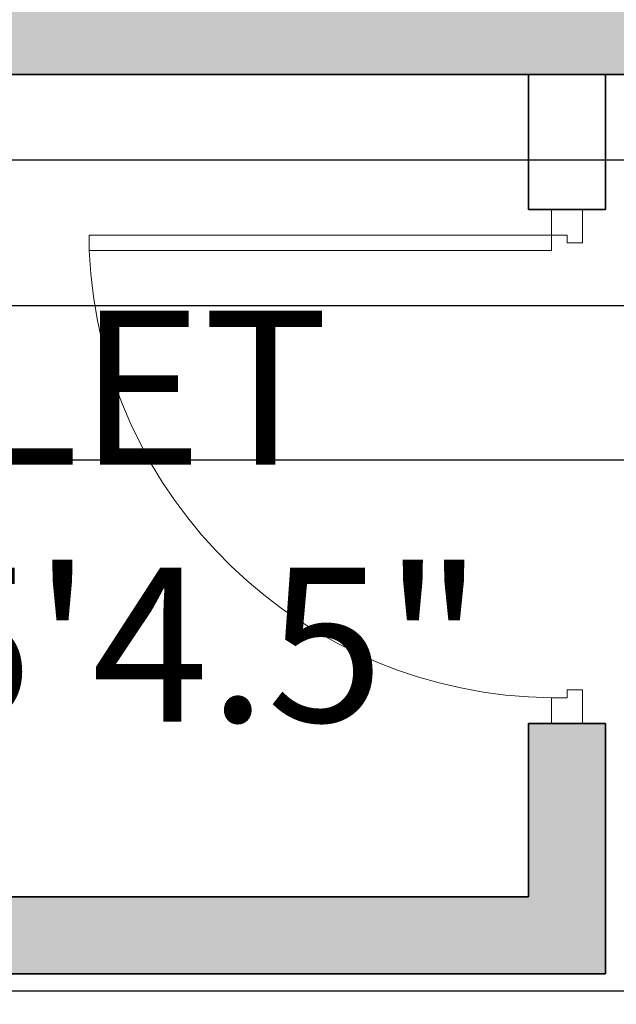
# Model space of a CAD drawing. Units: inches. Extents: x 2696 to 3240, y 1564 to 2310.
# Tile 21 of 76: x 2792 to 2827, y 1852 to 1910. Entities that reach past the tile are written whole.
import ezdxf

# ---------------------------------------------------------------- set-up
doc = ezdxf.new("R2010")
doc.units = ezdxf.units.IN
for name, color, linetype, lineweight in [('A-ANNO-DIMS', 3, 'Continuous', 18), ('A-AREA-IDEN', 7, 'Continuous', 18), ('A-DOOR', 4, 'Continuous', 18), ('A-WALL', 7, 'Continuous', 35), ('A-WALL-PATT', 9, 'Continuous', 13)]:
    doc.layers.add(name, color=color, linetype=linetype, lineweight=lineweight)
doc.styles.add('TIMES NEW', font='times.ttf')
doc.styles.add('YQ_DIM', font='SUPEROS.SHX', dxfattribs={"width": 0.8, "bigfont": 'HZDX.SHX'})
doc.dimstyles.new('Siddhuu', dxfattribs={"dimtxt": 6, "dimasz": 2.5, "dimexe": 1.25, "dimexo": 0.625, "dimtad": 1, "dimdec": 1, "dimlunit": 4, "dimtxsty": 'TIMES NEW', "dimcen": 2.5, "dimclrd": 256, "dimclre": 1, "dimclrt": 7, "dimadec": 0, "dimazin": 0, "dimtfac": 1, "dimtdec": 1, "dimtmove": 0, "dimatfit": 3, "dimfxl": 1, "dimtolj": 1, "dimlwd": -1, "dimarcsym": 0})

# ---------------------------------------------------------------- blocks, each defined once
blk = doc.blocks.new('DR_D01')
for p, q in [((-0.45, 0.93), (-0.42, 0.93)), ((-0.45, 0.03), (-0.45, 0.93)), ((-0.42, 0.03), (-0.42, 0.93)), ((-0.5, 0.03), (-0.42, 0.03)), ((-0.5, 0.03), (-0.5, -0.03)), ((-0.45, 0.03), (-0.45, 0)), ((0.45, 0.03), (0.45, 0)), ((0.5, 0.03), (0.45, 0.03)), ((0.5, -0.03), (0.5, 0.03)), ((-0.45, 0), (-0.435, 0)), ((-0.435, 0), (-0.435, -0.03)), ((0.435, 0), (0.435, -0.03)), ((0.45, 0), (0.435, 0)), ((-0.435, -0.03), (-0.5, -0.03)), ((0.435, -0.03), (0.5, -0.03))]:
    blk.add_line(p, q)
blk.add_arc((-0.4602, 0.0206), 0.9103, 0.5915, 87.4664)
blk = doc.blocks.new('*D55')
at = {"layer": 'A-ANNO-DIMS', "color": 1, "lineweight": -2, "transparency": 16777216}
for p, q in [((3189.986, 1980.201), (2709.361, 1980.201)), ((3189.986, 1893.201), (2709.361, 1893.201))]:
    blk.add_line(p, q, dxfattribs=at)
at = {"layer": 'A-ANNO-DIMS', "transparency": 16777216}
blk.add_line((2710.611, 1895.701), (2710.611, 1977.701), dxfattribs=at)
for points in [[(2710.195, 1977.701), (2711.028, 1977.701), (2710.611, 1980.201)], [(2710.195, 1895.701), (2711.028, 1895.701), (2710.611, 1893.201)]]:
    blk.add_solid(points, dxfattribs=at)
at = {"layer": 'Defpoints', "color": 0, "transparency": 16777216}
for p in [(2710.611, 1980.201), (3190.611, 1980.201), (3190.611, 1893.201)]:
    blk.add_point(p, dxfattribs=at)
at = {"layer": 'A-ANNO-DIMS', "color": 7, "transparency": 16777216, "insert": (2706.926, 1936.701), "char_height": 6, "attachment_point": 5, "rotation": 90, "style": 'TIMES NEW'}
blk.add_mtext('\\A1;7\'-3"', dxfattribs=at)
blk = doc.blocks.new('*D57')
at = {"layer": 'A-ANNO-DIMS', "color": 1, "lineweight": -2, "transparency": 16777216}
for p, q in [((2754.611, 2018.576), (2754.611, 1568.951)), ((2956.709, 2018.576), (2956.709, 1568.951))]:
    blk.add_line(p, q, dxfattribs=at)
at = {"layer": 'A-ANNO-DIMS', "transparency": 16777216}
blk.add_line((2757.111, 1570.201), (2954.209, 1570.201), dxfattribs=at)
for points in [[(2757.111, 1570.618), (2757.111, 1569.784), (2754.611, 1570.201)], [(2954.209, 1570.618), (2954.209, 1569.784), (2956.709, 1570.201)]]:
    blk.add_solid(points, dxfattribs=at)
at = {"layer": 'Defpoints', "color": 0, "transparency": 16777216}
for p in [(2754.611, 2019.201), (2956.709, 2019.201), (2956.709, 1570.201)]:
    blk.add_point(p, dxfattribs=at)
at = {"layer": 'A-ANNO-DIMS', "color": 7, "transparency": 16777216, "insert": (2855.66, 1573.878), "char_height": 6, "attachment_point": 5, "style": 'TIMES NEW'}
blk.add_mtext('\\A1;16\'-10"', dxfattribs=at)
blk = doc.blocks.new('*D78')
at = {"layer": 'A-ANNO-DIMS', "transparency": 16777216}
for p, q in [((2710.611, 1901.701), (2710.611, 1935.101)), ((2710.611, 1895.701), (2710.611, 1899.201))]:
    blk.add_line(p, q, dxfattribs=at)
at = {"layer": 'A-ANNO-DIMS', "color": 1, "lineweight": -2, "transparency": 16777216}
for p, q in [((3189.986, 1901.701), (2709.361, 1901.701)), ((3189.986, 1893.201), (2709.361, 1893.201))]:
    blk.add_line(p, q, dxfattribs=at)
at = {"layer": 'A-ANNO-DIMS', "transparency": 16777216}
for points in [[(2710.195, 1899.201), (2711.028, 1899.201), (2710.611, 1901.701)], [(2710.195, 1895.701), (2711.028, 1895.701), (2710.611, 1893.201)]]:
    blk.add_solid(points, dxfattribs=at)
at = {"layer": 'Defpoints', "color": 0, "transparency": 16777216}
for p in [(2710.611, 1901.701), (3190.611, 1901.701), (3190.611, 1893.201)]:
    blk.add_point(p, dxfattribs=at)
at = {"layer": 'A-ANNO-DIMS', "color": 7, "transparency": 16777216, "insert": (2706.85, 1919.651), "char_height": 6, "attachment_point": 5, "rotation": 90, "style": 'TIMES NEW'}
blk.add_mtext('\\A1;0\'-8 1/2"', dxfattribs=at)
blk = doc.blocks.new('*D79')
at = {"layer": 'A-ANNO-DIMS', "color": 1, "lineweight": -2, "transparency": 16777216}
for p, q in [((3189.986, 1884.201), (2709.361, 1884.201)), ((3189.986, 1853.201), (2709.361, 1853.201))]:
    blk.add_line(p, q, dxfattribs=at)
at = {"layer": 'A-ANNO-DIMS', "transparency": 16777216}
blk.add_line((2710.611, 1881.701), (2710.611, 1855.701), dxfattribs=at)
for points in [[(2710.195, 1881.701), (2711.028, 1881.701), (2710.611, 1884.201)], [(2710.195, 1855.701), (2711.028, 1855.701), (2710.611, 1853.201)]]:
    blk.add_solid(points, dxfattribs=at)
at = {"layer": 'Defpoints', "color": 0, "transparency": 16777216}
for p in [(3190.611, 1884.201), (2710.611, 1853.201), (3190.611, 1853.201)]:
    blk.add_point(p, dxfattribs=at)
at = {"layer": 'A-ANNO-DIMS', "color": 7, "transparency": 16777216, "insert": (2706.926, 1868.701), "char_height": 6, "attachment_point": 5, "rotation": 90, "style": 'TIMES NEW'}
blk.add_mtext('\\A1;2\'-7"', dxfattribs=at)

msp = doc.modelspace()

# ---------------------------------------------------------------- hatches: boundary and pattern name
at = {"layer": 'A-WALL-PATT', "transparency": 33554556}
h = msp.add_hatch(color=256, dxfattribs=at)
h.dxf.hatch_style = 1
h.paths.add_polyline_path([(2879.111, 2253.201), (2905.91, 2253.201), (2905.91, 2262.201), (2841.889, 2262.201), (2841.889, 2253.201), (2870.111, 2253.201), (2870.111, 2176.601), (2965.709, 2176.601), (2965.709, 2206.701), (2973.583, 2206.701), (2973.583, 2215.701), (2965.709, 2215.701), (2965.709, 2262.201), (2929.91, 2262.201), (2929.91, 2253.201), (2956.709, 2253.201), (2956.709, 2185.601), (2879.111, 2185.601)])
h.paths.add_polyline_path([(2782.834, 2262.201), (2745.611, 2262.201), (2745.611, 2228.729), (2754.611, 2228.729), (2754.611, 2253.201), (2782.834, 2253.201)])
h.paths.add_polyline_path([(2754.611, 2136.201), (2965.709, 2136.201), (2965.709, 2145.201), (2879.111, 2145.201), (2879.111, 2147.074), (2877.34, 2147.074), (2870.111, 2147.074), (2870.111, 2145.201), (2754.611, 2145.201), (2754.611, 2169.674), (2745.611, 2169.674), (2745.611, 2000.201), (2754.611, 2000.201), (2754.611, 2019.201), (2849.083, 2019.201), (2849.083, 2023.701), (2841.209, 2023.701), (2841.209, 2051.827), (2836.709, 2051.827), (2836.709, 2023.701), (2754.611, 2023.701), (2754.611, 2091.201), (2836.709, 2091.201), (2836.709, 2087.827), (2841.209, 2087.827), (2841.209, 2095.701), (2754.611, 2095.701)])
h.paths.add_polyline_path([(2965.709, 2136.201), (2956.709, 2136.201), (2956.709, 2023.701), (2885.083, 2023.701), (2885.083, 2019.201), (2956.709, 2019.201), (2956.709, 1950.575), (2965.709, 1950.575), (2965.709, 1980.201), (2973.583, 1980.201), (2973.583, 1989.201), (2965.709, 1989.201)])
h.paths.add_polyline_path([(2754.611, 1906.701), (2880.209, 1906.701), (2884.709, 1906.701), (2956.709, 1906.701), (2956.709, 1792.701), (2944.709, 1792.701), (2944.709, 1783.701), (2956.709, 1783.701), (2956.709, 1740.201), (2884.709, 1740.201), (2884.709, 1783.701), (2896.709, 1783.701), (2896.709, 1792.701), (2884.709, 1792.701), (2884.709, 1846.701), (2880.209, 1846.701), (2880.209, 1740.201), (2754.611, 1740.201), (2754.611, 1777.201), (2745.611, 1777.201), (2745.611, 1692.701), (2754.611, 1692.701), (2754.611, 1731.201), (2956.709, 1731.201), (2956.709, 1723.327), (2965.709, 1723.327), (2965.709, 1884.201), (2973.583, 1884.201), (2973.583, 1893.201), (2965.709, 1893.201), (2965.709, 1914.575), (2956.709, 1914.575), (2956.709, 1911.201), (2754.611, 1911.201), (2754.611, 1930.201), (2745.611, 1930.201), (2745.611, 1817.201), (2754.611, 1817.201), (2754.611, 1854.201), (2826.611, 1854.201), (2826.611, 1868.827), (2822.111, 1868.827), (2822.111, 1858.701), (2754.611, 1858.701)])
h.paths.add_polyline_path([(2965.709, 1656.201), (3008.237, 1656.201), (3008.237, 1665.201), (2965.709, 1665.201), (2965.709, 1693.327), (2956.709, 1693.327), (2956.709, 1686.201), (2934.583, 1686.201), (2934.583, 1681.701), (2956.709, 1681.701), (2956.709, 1614.201), (2896.709, 1614.201), (2896.709, 1681.701), (2904.583, 1681.701), (2904.583, 1686.201), (2892.209, 1686.201), (2892.209, 1614.201), (2858.41, 1614.201), (2858.41, 1605.201), (2965.709, 1605.201)])
h.paths.add_polyline_path([(2788.41, 1614.201), (2754.611, 1614.201), (2754.611, 1652.701), (2745.611, 1652.701), (2745.611, 1605.201), (2788.41, 1605.201)])
h.paths.add_polyline_path([(3199.611, 1633.048), (3190.611, 1633.048), (3190.611, 1614.201), (3082.611, 1614.201), (3082.611, 1665.201), (3070.237, 1665.201), (3070.237, 1656.201), (3078.111, 1656.201), (3078.111, 1605.201), (3199.611, 1605.201)])
h.paths.add_polyline_path([(3199.611, 1702.048), (3190.611, 1702.048), (3190.611, 1699.701), (3106.611, 1699.701), (3106.611, 1747.701), (3190.611, 1747.701), (3190.611, 1752.201), (3082.611, 1752.201), (3082.611, 1760.075), (3078.111, 1760.075), (3078.111, 1747.701), (3102.111, 1747.701), (3102.111, 1699.701), (3078.111, 1699.701), (3078.111, 1695.201), (3190.611, 1695.201), (3190.611, 1676.355), (3199.611, 1676.355)])
h.paths.add_polyline_path([(3199.611, 1783.201), (3190.611, 1783.201), (3190.611, 1745.355), (3199.611, 1745.355)])
h.paths.add_polyline_path([(3082.611, 1884.201), (3190.611, 1884.201), (3190.611, 1853.201), (3199.611, 1853.201), (3199.611, 1901.701), (3190.611, 1901.701), (3190.611, 1893.201), (3005.583, 1893.201), (3005.583, 1891.281), (3005.583, 1884.201), (3078.111, 1884.201), (3078.111, 1792.075), (3082.611, 1792.075)])
h.paths.add_polyline_path([(3199.611, 1994.701), (3190.611, 1994.701), (3190.611, 1989.201), (3073.709, 1989.201), (3073.709, 2034.201), (3069.209, 2034.201), (3069.209, 1989.201), (3005.583, 1989.201), (3005.583, 1980.201), (3190.611, 1980.201), (3190.611, 1971.701), (3199.611, 1971.701)])
h.paths.add_polyline_path([(3199.611, 2155.201), (3190.611, 2155.201), (3190.611, 2064.701), (3199.611, 2064.701)])
h.paths.add_polyline_path([(3190.611, 2074.701), (3106.611, 2074.701), (3106.611, 2122.701), (3190.611, 2122.701), (3190.611, 2127.201), (3082.709, 2127.201), (3082.709, 2135.075), (3073.709, 2135.075), (3073.709, 2122.701), (3102.111, 2122.701), (3102.111, 2074.701), (3069.209, 2074.701), (3069.209, 2070.201), (3190.611, 2070.201)])
h.paths.add_polyline_path([(3082.709, 2253.201), (3190.611, 2253.201), (3190.611, 2225.201), (3199.611, 2225.201), (3199.611, 2262.201), (3073.709, 2262.201), (3073.709, 2215.701), (3035.583, 2215.701), (3035.583, 2206.701), (3073.709, 2206.701), (3073.709, 2171.075), (3082.709, 2171.075)])

# ---------------------------------------------------------------- linework, layer by layer
at = {"layer": 'A-WALL'}
for p, q in [((2754.611, 1906.701), (2880.209, 1906.701)), ((2822.111, 1898.827), (2822.111, 1906.701)), ((2826.611, 1898.827), (2826.611, 1906.701)), ((2822.111, 1898.827), (2826.611, 1898.827)), ((2822.111, 1858.701), (2822.111, 1868.827)), ((2822.111, 1868.827), (2826.611, 1868.827)), ((2826.611, 1854.201), (2826.611, 1868.827)), ((2754.611, 1858.701), (2822.111, 1858.701)), ((2754.611, 1854.201), (2826.611, 1854.201))]:
    msp.add_line(p, q, dxfattribs=at)

# ---------------------------------------------------------------- block references
at = {"layer": 'A-DOOR', "xscale": 30, "yscale": -30, "zscale": 30, "rotation": 270}
msp.add_blockref('DR_D01', (2824.361, 1883.827), dxfattribs=at)

# ---------------------------------------------------------------- texts
at = {"layer": 'A-AREA-IDEN', "insert": (2769.129, 1892.921), "char_height": 9, "attachment_point": 1, "style": 'YQ_DIM'}
msp.add_mtext_dynamic_manual_height_columns('TOILET\\P5\'X5\'4.5"', width=48.00324, gutter_width=12.5, heights=[0], dxfattribs=at)

# ---------------------------------------------------------------- dimensions: what is measured, and where the dimension line sits
at = {"layer": 'A-ANNO-DIMS'}
dim = msp.add_linear_dim(base=(2956.709, 1570.201), p1=(2754.611, 2019.201), p2=(2956.709, 2019.201), dimstyle='Siddhuu', override={"dimdec": 1, "dimlfac": 1, "dimrnd": 0, "dimzin": 1, "dimdsep": 46, "dimlunit": 4, "dimfrac": 2}, dxfattribs=at)
dim.commit()
dim.dimension.update_dxf_attribs({"geometry": '*D57', "text_midpoint": (2855.66, 1573.878)})
for base, p1, p2, picture, middle in [((2710.611, 1980.201), (3190.611, 1893.201), (3190.611, 1980.201), '*D55', (2706.926, 1936.701)), ((2710.611, 1901.701), (3190.611, 1893.201), (3190.611, 1901.701), '*D78', (2706.85, 1919.651)), ((2710.611, 1853.201), (3190.611, 1884.201), (3190.611, 1853.201), '*D79', (2706.926, 1868.701))]:
    dim = msp.add_linear_dim(base=base, p1=p1, p2=p2, angle=90, dimstyle='Siddhuu', override={"dimdec": 1, "dimlfac": 1, "dimrnd": 0, "dimzin": 1, "dimdsep": 46, "dimlunit": 4, "dimfrac": 2}, dxfattribs=at)
    dim.commit()
    dim.dimension.update_dxf_attribs({"geometry": picture, "text_midpoint": middle})

doc.saveas('drawing.dxf')
